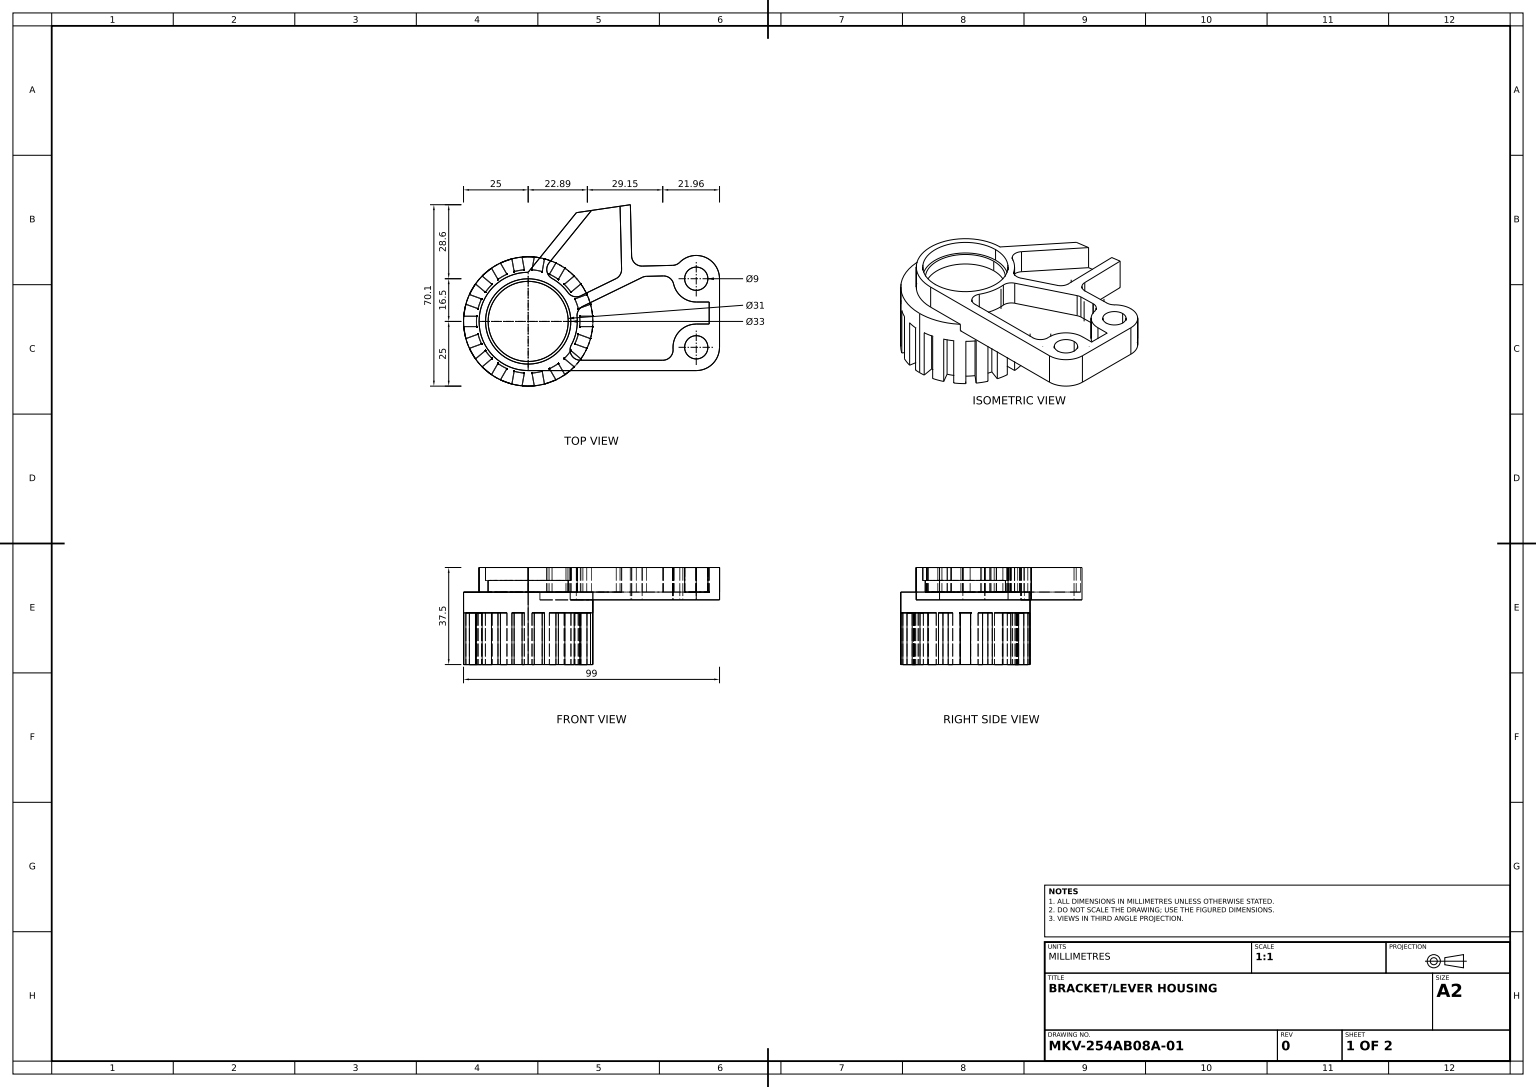
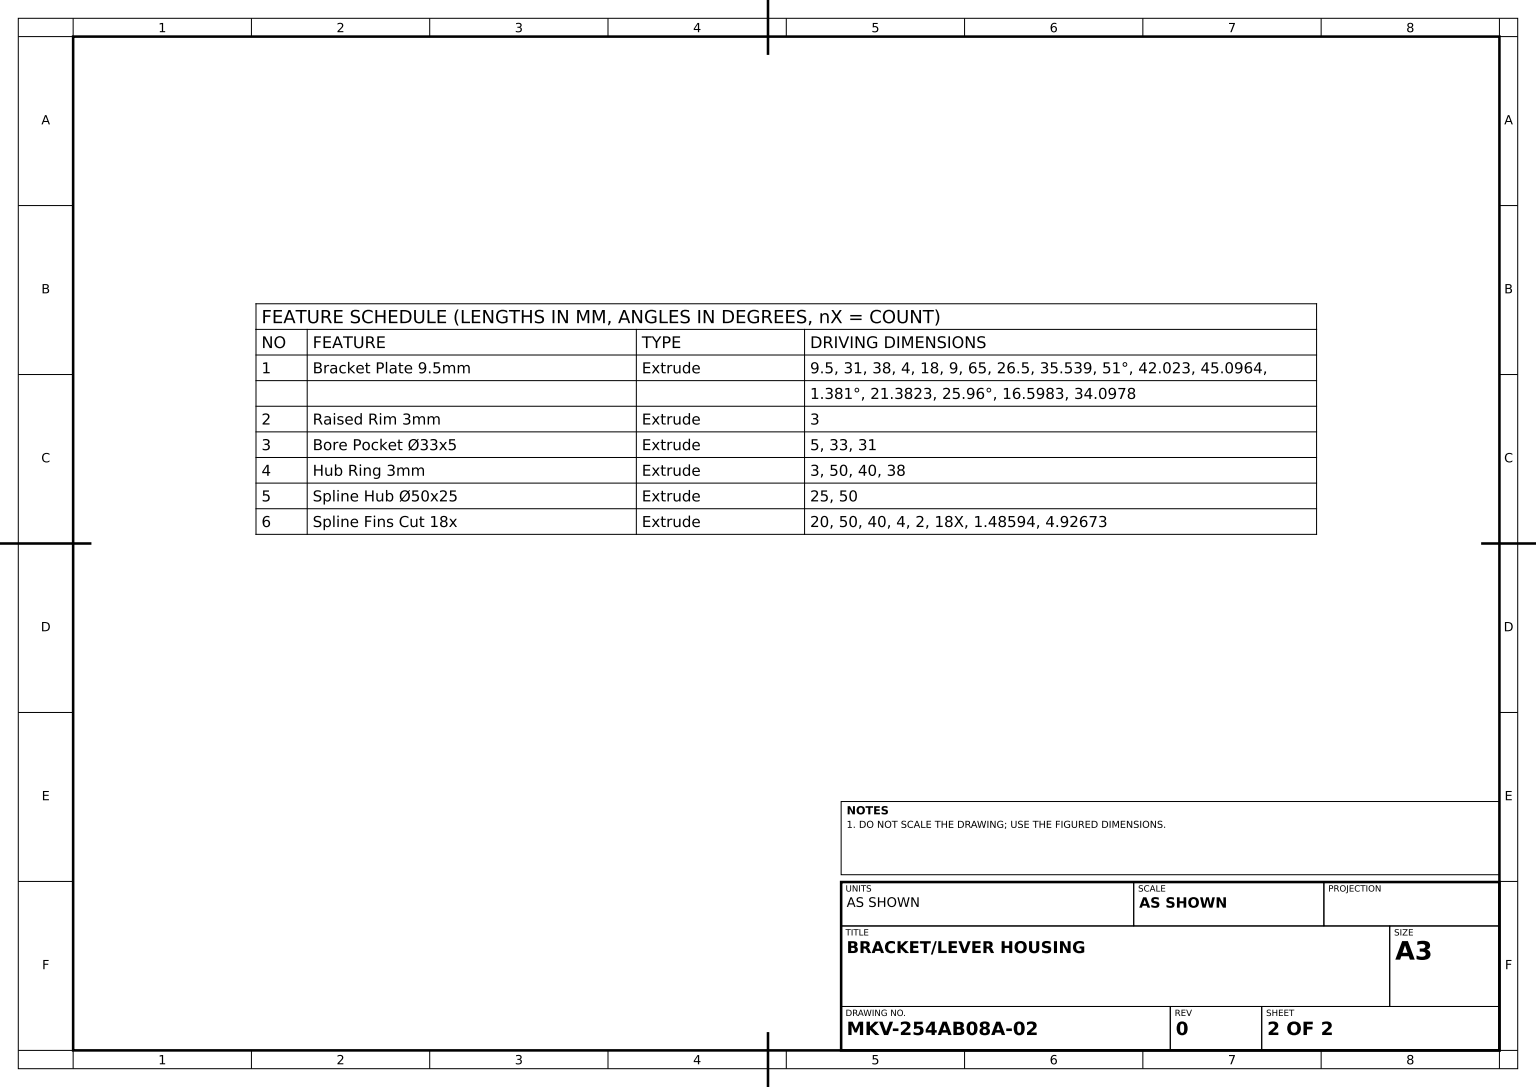
from build123d import *
from build123d.topology import SkipClean

# Parameters (mm, degrees)
BRACKET_PLATE_PROFILE_R   = 15.5
BRACKET_PLATE_PROFILE_R_2 = 4.5
BRACKET_PLATE_9_5MM_DEPTH = 9.5
RAISED_START              = 3
RAISED_RIM_PROFILE_R      = 15.5
RAISED_RIM_PROFILE_R_2    = 4.5
RAISED_RIM_3MM_DEPTH      = 3
BORE_START                = -5
BORE_POCKET_PROFILE_R     = 16.5
BORE_POCKET_PROFILE_R_2   = 15.5
BORE_POCKET_33X5_DEPTH    = 5
HUB_RING_3MM_DEPTH        = 3
SPLINE_START              = 25
HUB_PROFILE_50_R          = 25
SPLINE_HUB_50X25_DEPTH    = 25
SPLINE_FINS_CUT_18X_DEPTH = 20


with BuildPart() as part:
    # Bracket Plate Profile → Bracket Plate 9.5mm (new body)
    with BuildSketch(Plane(origin=(0, 0, 0), x_dir=(1, 0, 0), z_dir=(0, 1, 0))):
        with BuildLine():
            Line((18.643636366, 42.022973535), (0, 19))
            ThreePointArc((0, 19), (-19, 0), (0, -19))
            Line((0, -19), (65, -19))
            ThreePointArc((65, -19), (71.363961031, -16.363961031), (74, -10))
            Line((74, -10), (74, 16.5))
            ThreePointArc((74, 16.5), (68.431859925, 24.819996241), (58.617258344, 22.845124818))
            ThreePointArc((58.617258344, 22.845124818), (57.361084073, 21.990713763), (55.876909068, 21.666342679))
            Line((55.876909068, 21.666342679), (44.099015371, 21.382339908))
            ThreePointArc((44.099015371, 21.382339908), (41.243168009, 22.485389703), (40.003752964, 25.284752729))
            Line((40.003752964, 25.284752729), (39.526030045, 45.096424793))
            Line((39.526030045, 45.096424793), (35.539017067, 44.509619935))
            Line((35.539017067, 44.509619935), (36.125791513, 20.175466313))
            ThreePointArc((36.125791513, 20.175466313), (35.606668042, 18.10633032), (34.097824063, 16.598284304))
            Line((34.097824063, 16.598284304), (20.364841939, 9.913284663))
            ThreePointArc((20.364841939, 9.913284663), (17.643973229, 9.629232951), (15.376876038, 11.160272546))
            ThreePointArc((15.376876038, 11.160272546), (12.604877523, 14.216788056), (9.23838051, 16.602780657))
            ThreePointArc((9.23838051, 16.602780657), (7.256175018, 19.338058171), (8.074718877, 22.615384465))
            Line((8.074718877, 22.615384465), (24.487120066, 42.883012025))
            Line((24.487120066, 42.883012025), (18.643636366, 42.022973535))
        make_face()
        with Locations(Location((0, 0, 0), (0, 0, 270))):
            Circle(BRACKET_PLATE_PROFILE_R, mode=Mode.SUBTRACT)
        with Locations(Location((65, -10, 0), (0, 0, 270))):
            Circle(BRACKET_PLATE_PROFILE_R_2, mode=Mode.SUBTRACT)
        with BuildLine():
            Line((65, 7.5), (70, 7.5))
            Line((70, 7.5), (70, -1))
            Line((70, -1), (65, -1))
            ThreePointArc((65, -1), (58.395805529, -3.885704016), (56.026666725, -10.692307692))
            ThreePointArc((56.026666725, -10.692307692), (54.973716146, -13.717464882), (52.038518603, -15))
            Line((52.038518603, -15), (20.199009877, -15))
            ThreePointArc((20.199009877, -15), (16.760102062, -13.043015674), (16.686138594, -9.086956522))
            ThreePointArc((16.686138594, -9.086956522), (18.61955403, -3.783147859), (18.909266102, 1.854630825))
            ThreePointArc((18.909266102, 1.854630825), (19.399195242, 4.197804576), (21.139435388, 5.841598366))
            Line((21.139435388, 5.841598366), (44.100719397, 17.018790179))
            ThreePointArc((44.100719397, 17.018790179), (44.906218523, 17.308984599), (45.755023444, 17.421108847))
            Line((45.755023444, 17.421108847), (52.236091905, 17.577388182))
            ThreePointArc((52.236091905, 17.577388182), (54.785023693, 16.73848877), (56.230203867, 14.477458086))
            ThreePointArc((56.230203867, 14.477458086), (59.396558077, 9.457171121), (65, 7.5))
        make_face(mode=Mode.SUBTRACT)
        with Locations(Location((65, 16.5, 0), (0, 0, 270))):
            Circle(BRACKET_PLATE_PROFILE_R_2, mode=Mode.SUBTRACT)
    extrude(amount=BRACKET_PLATE_9_5MM_DEPTH)

    # Raised Rim Profile → Raised Rim 3mm (add)
    # profile 1 of 8: a face of its own
    with SkipClean():  # the faces are left unmerged after this step: merging them gives an invalid solid
        with BuildSketch(Plane.XZ.offset(RAISED_START)):
            with BuildLine():
                ThreePointArc((16.686138594, 9.086956522), (9.704324451, 16.334812119), (0, 19))
                ThreePointArc((0, 19), (-19, 0), (0, -19))
                ThreePointArc((0, -19), (4.772167616, -18.39093299), (9.23838051, -16.602780657))
                ThreePointArc((9.23838051, -16.602780657), (12.604877523, -14.216788056), (15.376876038, -11.160272546))
                ThreePointArc((15.376876038, -11.160272546), (17.763266244, -6.742875672), (18.909266102, -1.854630825))
                ThreePointArc((18.909266102, -1.854630825), (18.977302969, -0.92842449), (19, 0))
                ThreePointArc((19, 0), (18.412450045, 4.688462793), (16.686138594, 9.086956522))
            make_face()
            with Locations(Location((0, 0, 0), (0, 0, 90))):
                Circle(RAISED_RIM_PROFILE_R, mode=Mode.SUBTRACT)
        # profile 2 of 8: a face of its own
        with BuildSketch(Plane.XZ.offset(RAISED_START)):
            with Locations(Location((0, 0, 0), (0, 0, 90))):
                Circle(RAISED_RIM_PROFILE_R)
        # profile 3 of 8: a face of its own
        with BuildSketch(Plane.XZ.offset(RAISED_START)):
            with BuildLine():
                Line((65, 19), (0, 19))
                ThreePointArc((0, 19), (9.704324451, 16.334812119), (16.686138594, 9.086956522))
                ThreePointArc((16.686138594, 9.086956522), (16.760102062, 13.043015674), (20.199009877, 15))
                Line((20.199009877, 15), (52.038518603, 15))
                ThreePointArc((52.038518603, 15), (54.973716146, 13.717464882), (56.026666725, 10.692307692))
                ThreePointArc((56.026666725, 10.692307692), (58.395805529, 3.885704016), (65, 1))
                Line((65, 1), (70, 1))
                Line((70, 1), (70, -7.5))
                Line((70, -7.5), (65, -7.5))
                ThreePointArc((65, -7.5), (59.396558077, -9.457171121), (56.230203867, -14.477458086))
                ThreePointArc((56.230203867, -14.477458086), (54.785023693, -16.73848877), (52.236091905, -17.577388182))
                Line((52.236091905, -17.577388182), (45.755023444, -17.421108847))
                ThreePointArc((45.755023444, -17.421108847), (44.906218523, -17.308984599), (44.100719397, -17.018790179))
                Line((44.100719397, -17.018790179), (21.139435388, -5.841598366))
                ThreePointArc((21.139435388, -5.841598366), (19.399195242, -4.197804576), (18.909266102, -1.854630825))
                ThreePointArc((18.909266102, -1.854630825), (17.763266244, -6.742875672), (15.376876038, -11.160272546))
                ThreePointArc((15.376876038, -11.160272546), (17.643973229, -9.629232951), (20.364841939, -9.913284663))
                Line((20.364841939, -9.913284663), (34.097824063, -16.598284304))
                ThreePointArc((34.097824063, -16.598284304), (35.606668042, -18.10633032), (36.125791513, -20.175466313))
                Line((36.125791513, -20.175466313), (35.539017067, -44.509619935))
                Line((35.539017067, -44.509619935), (39.526030045, -45.096424793))
                Line((39.526030045, -45.096424793), (40.003752964, -25.284752729))
                ThreePointArc((40.003752964, -25.284752729), (41.243168009, -22.485389703), (44.099015371, -21.382339908))
                Line((44.099015371, -21.382339908), (55.876909068, -21.666342679))
                ThreePointArc((55.876909068, -21.666342679), (57.361084073, -21.990713763), (58.617258344, -22.845124818))
                ThreePointArc((58.617258344, -22.845124818), (68.431859925, -24.819996241), (74, -16.5))
                Line((74, -16.5), (74, 10))
                ThreePointArc((74, 10), (71.363961031, 16.363961031), (65, 19))
            make_face()
            with Locations(Location((65, -16.5, 0), (0, 0, 90))):
                Circle(RAISED_RIM_PROFILE_R_2, mode=Mode.SUBTRACT)
            with Locations(Location((65, 10, 0), (0, 0, 90))):
                Circle(RAISED_RIM_PROFILE_R_2, mode=Mode.SUBTRACT)
        # profile 4 of 8: a face of its own
        with BuildSketch(Plane.XZ.offset(RAISED_START)):
            with Locations(Location((65, 10, 0), (0, 0, 90))):
                Circle(RAISED_RIM_PROFILE_R_2)
        # profile 5 of 8: a face of its own
        with BuildSketch(Plane.XZ.offset(RAISED_START)):
            with Locations(Location((65, -16.5, 0), (0, 0, 90))):
                Circle(RAISED_RIM_PROFILE_R_2)
        # profile 6 of 8: a face of its own
        with BuildSketch(Plane.XZ.offset(RAISED_START)):
            with BuildLine():
                ThreePointArc((16.686138594, 9.086956522), (16.760102062, 13.043015674), (20.199009877, 15))
                Line((20.199009877, 15), (52.038518603, 15))
                ThreePointArc((52.038518603, 15), (54.973716146, 13.717464882), (56.026666725, 10.692307692))
                ThreePointArc((56.026666725, 10.692307692), (58.395805529, 3.885704016), (65, 1))
                Line((65, 1), (70, 1))
                Line((70, 1), (70, -7.5))
                Line((70, -7.5), (65, -7.5))
                ThreePointArc((65, -7.5), (59.396558077, -9.457171121), (56.230203867, -14.477458086))
                ThreePointArc((56.230203867, -14.477458086), (54.785023693, -16.73848877), (52.236091905, -17.577388182))
                Line((52.236091905, -17.577388182), (45.755023444, -17.421108847))
                ThreePointArc((45.755023444, -17.421108847), (44.906218523, -17.308984599), (44.100719397, -17.018790179))
                Line((44.100719397, -17.018790179), (21.139435388, -5.841598366))
                ThreePointArc((21.139435388, -5.841598366), (19.399195242, -4.197804576), (18.909266102, -1.854630825))
                ThreePointArc((18.909266102, -1.854630825), (18.61955403, 3.783147859), (16.686138594, 9.086956522))
            make_face()
        # profile 7 of 8: a face of its own
        with BuildSketch(Plane.XZ.offset(RAISED_START)):
            with BuildLine():
                ThreePointArc((15.376876038, -11.160272546), (12.604877523, -14.216788056), (9.23838051, -16.602780657))
                ThreePointArc((9.23838051, -16.602780657), (7.256175018, -19.338058171), (8.074718877, -22.615384465))
                Line((8.074718877, -22.615384465), (24.487120066, -42.883012025))
                Line((24.487120066, -42.883012025), (35.539017067, -44.509619935))
                Line((35.539017067, -44.509619935), (36.125791513, -20.175466313))
                ThreePointArc((36.125791513, -20.175466313), (35.606668042, -18.10633032), (34.097824063, -16.598284304))
                Line((34.097824063, -16.598284304), (20.364841939, -9.913284663))
                ThreePointArc((20.364841939, -9.913284663), (17.643973229, -9.629232951), (15.376876038, -11.160272546))
            make_face()
        # profile 8 of 8: a face of its own
        with BuildSketch(Plane.XZ.offset(RAISED_START)):
            with BuildLine():
                ThreePointArc((9.23838051, -16.602780657), (4.772167616, -18.39093299), (0, -19))
                Line((0, -19), (18.643636366, -42.022973535))
                Line((18.643636366, -42.022973535), (24.487120066, -42.883012025))
                Line((24.487120066, -42.883012025), (8.074718877, -22.615384465))
                ThreePointArc((8.074718877, -22.615384465), (7.256175018, -19.338058171), (9.23838051, -16.602780657))
            make_face()
        extrude(amount=-RAISED_RIM_3MM_DEPTH)

    # Bore Pocket Profile → Bore Pocket Ø33x5 (cut)
    with SkipClean():  # the faces are left unmerged after this step: merging them gives an invalid solid
        with BuildSketch(Plane(origin=(0, 9.5, 0), x_dir=(1, 0, 0), z_dir=(0, 1, 0)).offset(BORE_START)):
            with Locations(Location((0, 0, 0), (0, 0, 270))):
                Circle(BORE_POCKET_PROFILE_R)
            with Locations(Location((0, 0, 0), (0, 0, 270))):
                Circle(BORE_POCKET_PROFILE_R_2, mode=Mode.SUBTRACT)
        extrude(amount=BORE_POCKET_33X5_DEPTH, mode=Mode.SUBTRACT)

    # Hub Ring Profile → Hub Ring 3mm (add)
    with BuildSketch(Plane.XZ.offset(3)):
        with BuildLine():
            Line((0, 19), (6.244997998, 19))
            ThreePointArc((6.244997998, 19), (-19.807511084, 2.768122951), (0.796921894, -19.98411658))
            Line((0.796921894, -19.98411658), (0, -19))
            ThreePointArc((0, -19), (-19, 0), (0, 19))
        make_face()
        with BuildLine():
            ThreePointArc((4.524413475, -24.587185335), (19.210808636, -15.998275893), (25, 0))
            ThreePointArc((25, 0), (22.706848309, 10.459399595), (16.248076809, 19))
            Line((16.248076809, 19), (6.244997998, 19))
            ThreePointArc((6.244997998, 19), (16.200308021, 11.728172066), (20, 0))
            ThreePointArc((20, 0), (14.421137921, -13.857517132), (0.796921894, -19.98411658))
            Line((0.796921894, -19.98411658), (4.524413475, -24.587185335))
        make_face()
        with BuildLine():
            Line((6.244997998, 19), (16.248076809, 19))
            ThreePointArc((16.248076809, 19), (-24.141971119, 6.493475994), (4.524413475, -24.587185335))
            Line((4.524413475, -24.587185335), (0.796921894, -19.98411658))
            ThreePointArc((0.796921894, -19.98411658), (-19.807511084, 2.768122951), (6.244997998, 19))
        make_face()
    extrude(amount=-HUB_RING_3MM_DEPTH)

    # Hub Profile Ø50 → Spline Hub Ø50x25 (add)
    with BuildSketch(Plane.XZ.offset(3).offset(SPLINE_START)):
        with Locations(Location((0, 0, 0), (0, 0, 270))):
            Circle(HUB_PROFILE_50_R)
    extrude(amount=-SPLINE_HUB_50X25_DEPTH)

    # Spline Fin Profile 18x → Spline Fins Cut 18x (cut)
    with BuildSketch(Plane.XZ.offset(28)):
        with BuildLine():
            ThreePointArc((-24.919871589, 2), (-25, 0), (-24.919871589, -2))
            Line((-24.919871589, -2), (-19.899748742, -2))
            ThreePointArc((-19.899748742, -2), (-20, 0), (-19.899748742, 2))
            Line((-19.899748742, 2), (-24.919871589, 2))
        make_face()
        with BuildLine():
            ThreePointArc((-24.10105973, -6.643712811), (-23.49231552, -8.550503583), (-22.732979156, -10.402483294))
            Line((-22.732979156, -10.402483294), (-18.015606762, -8.685500159))
            ThreePointArc((-18.015606762, -8.685500159), (-18.793852416, -6.840402867), (-19.383687335, -4.926729675))
            Line((-19.383687335, -4.926729675), (-24.10105973, -6.643712811))
        make_face()
        with BuildLine():
            ThreePointArc((-20.375304373, -14.486095806), (-19.151111078, -16.069690242), (-17.804153934, -17.550273578))
            Line((-17.804153934, -17.550273578), (-13.958516724, -14.323400814))
            ThreePointArc((-13.958516724, -14.323400814), (-15.320888862, -12.855752194), (-16.529667163, -11.259223041))
            Line((-16.529667163, -11.259223041), (-20.375304373, -14.486095806))
        make_face()
        with BuildLine():
            ThreePointArc((-14.191986602, -20.581241855), (-12.5, -21.650635095), (-10.727884987, -22.581241855))
            Line((-10.727884987, -22.581241855), (-8.217823563, -18.23368794))
            ThreePointArc((-8.217823563, -18.23368794), (-10, -17.320508076), (-11.681925179, -16.23368794))
            Line((-11.681925179, -16.23368794), (-14.191986602, -20.581241855))
        make_face()
        with BuildLine():
            ThreePointArc((-6.296905795, -24.193986389), (-4.341204442, -24.620193825), (-2.357674783, -24.8885791))
            Line((-2.357674783, -24.8885791), (-1.485939599, -19.9447232))
            ThreePointArc((-1.485939599, -19.9447232), (-3.472963553, -19.69615506), (-5.425170611, -19.250130489))
            Line((-5.425170611, -19.250130489), (-6.296905795, -24.193986389))
        make_face()
        with BuildLine():
            ThreePointArc((2.357674783, -24.8885791), (4.341204442, -24.620193825), (6.296905795, -24.193986389))
            Line((6.296905795, -24.193986389), (5.425170611, -19.250130489))
            ThreePointArc((5.425170611, -19.250130489), (3.472963553, -19.69615506), (1.485939599, -19.9447232))
            Line((1.485939599, -19.9447232), (2.357674783, -24.8885791))
        make_face()
        with BuildLine():
            ThreePointArc((10.727884987, -22.581241855), (12.5, -21.650635095), (14.191986602, -20.581241855))
            Line((14.191986602, -20.581241855), (11.681925179, -16.23368794))
            ThreePointArc((11.681925179, -16.23368794), (10, -17.320508076), (8.217823563, -18.23368794))
            Line((8.217823563, -18.23368794), (10.727884987, -22.581241855))
        make_face()
        with BuildLine():
            ThreePointArc((17.804153934, -17.550273578), (19.151111078, -16.069690242), (20.375304373, -14.486095806))
            Line((20.375304373, -14.486095806), (16.529667163, -11.259223041))
            ThreePointArc((16.529667163, -11.259223041), (15.320888862, -12.855752194), (13.958516724, -14.323400814))
            Line((13.958516724, -14.323400814), (17.804153934, -17.550273578))
        make_face()
        with BuildLine():
            Line((24.10105973, -6.643712811), (19.383687335, -4.926729675))
            ThreePointArc((19.383687335, -4.926729675), (18.793852416, -6.840402867), (18.015606762, -8.685500159))
            Line((18.015606762, -8.685500159), (22.732979156, -10.402483294))
            ThreePointArc((22.732979156, -10.402483294), (23.49231552, -8.550503583), (24.10105973, -6.643712811))
        make_face()
        with BuildLine():
            Line((19.899748742, -2), (24.919871589, -2))
            ThreePointArc((24.919871589, -2), (24.979959865, -1.000802248), (25, 0))
            ThreePointArc((25, 0), (24.979959865, 1.000802248), (24.919871589, 2))
            Line((24.919871589, 2), (19.899748742, 2))
            ThreePointArc((19.899748742, 2), (20, 0), (19.899748742, -2))
        make_face()
        with BuildLine():
            Line((19.383687335, 4.926729675), (24.10105973, 6.643712811))
            ThreePointArc((24.10105973, 6.643712811), (23.49231552, 8.550503583), (22.732979156, 10.402483294))
            Line((22.732979156, 10.402483294), (18.015606762, 8.685500159))
            ThreePointArc((18.015606762, 8.685500159), (18.793852416, 6.840402867), (19.383687335, 4.926729675))
        make_face()
        with BuildLine():
            Line((16.529667163, 11.259223041), (20.375304373, 14.486095806))
            ThreePointArc((20.375304373, 14.486095806), (19.151111078, 16.069690242), (17.804153934, 17.550273578))
            Line((17.804153934, 17.550273578), (13.958516724, 14.323400814))
            ThreePointArc((13.958516724, 14.323400814), (15.320888862, 12.855752194), (16.529667163, 11.259223041))
        make_face()
        with BuildLine():
            Line((11.681925179, 16.23368794), (14.191986602, 20.581241855))
            ThreePointArc((14.191986602, 20.581241855), (12.5, 21.650635095), (10.727884987, 22.581241855))
            Line((10.727884987, 22.581241855), (8.217823563, 18.23368794))
            ThreePointArc((8.217823563, 18.23368794), (10, 17.320508076), (11.681925179, 16.23368794))
        make_face()
        with BuildLine():
            Line((5.425170611, 19.250130489), (6.296905795, 24.193986389))
            ThreePointArc((6.296905795, 24.193986389), (4.341204442, 24.620193825), (2.357674783, 24.8885791))
            Line((2.357674783, 24.8885791), (1.485939599, 19.9447232))
            ThreePointArc((1.485939599, 19.9447232), (3.472963553, 19.69615506), (5.425170611, 19.250130489))
        make_face()
        with BuildLine():
            Line((-1.485939599, 19.9447232), (-2.357674783, 24.8885791))
            ThreePointArc((-2.357674783, 24.8885791), (-4.341204442, 24.620193825), (-6.296905795, 24.193986389))
            Line((-6.296905795, 24.193986389), (-5.425170611, 19.250130489))
            ThreePointArc((-5.425170611, 19.250130489), (-3.472963553, 19.69615506), (-1.485939599, 19.9447232))
        make_face()
        with BuildLine():
            Line((-8.217823563, 18.23368794), (-10.727884987, 22.581241855))
            ThreePointArc((-10.727884987, 22.581241855), (-12.5, 21.650635095), (-14.191986602, 20.581241855))
            Line((-14.191986602, 20.581241855), (-11.681925179, 16.23368794))
            ThreePointArc((-11.681925179, 16.23368794), (-10, 17.320508076), (-8.217823563, 18.23368794))
        make_face()
        with BuildLine():
            Line((-13.958516724, 14.323400814), (-17.804153934, 17.550273578))
            ThreePointArc((-17.804153934, 17.550273578), (-19.151111078, 16.069690242), (-20.375304373, 14.486095806))
            Line((-20.375304373, 14.486095806), (-16.529667163, 11.259223041))
            ThreePointArc((-16.529667163, 11.259223041), (-15.320888862, 12.855752194), (-13.958516724, 14.323400814))
        make_face()
        with BuildLine():
            ThreePointArc((-22.732979156, 10.402483294), (-23.49231552, 8.550503583), (-24.10105973, 6.643712811))
            Line((-24.10105973, 6.643712811), (-19.383687335, 4.926729675))
            ThreePointArc((-19.383687335, 4.926729675), (-18.793852416, 6.840402867), (-18.015606762, 8.685500159))
            Line((-18.015606762, 8.685500159), (-22.732979156, 10.402483294))
        make_face()
    extrude(amount=-SPLINE_FINS_CUT_18X_DEPTH, mode=Mode.SUBTRACT)


solid = part.part
